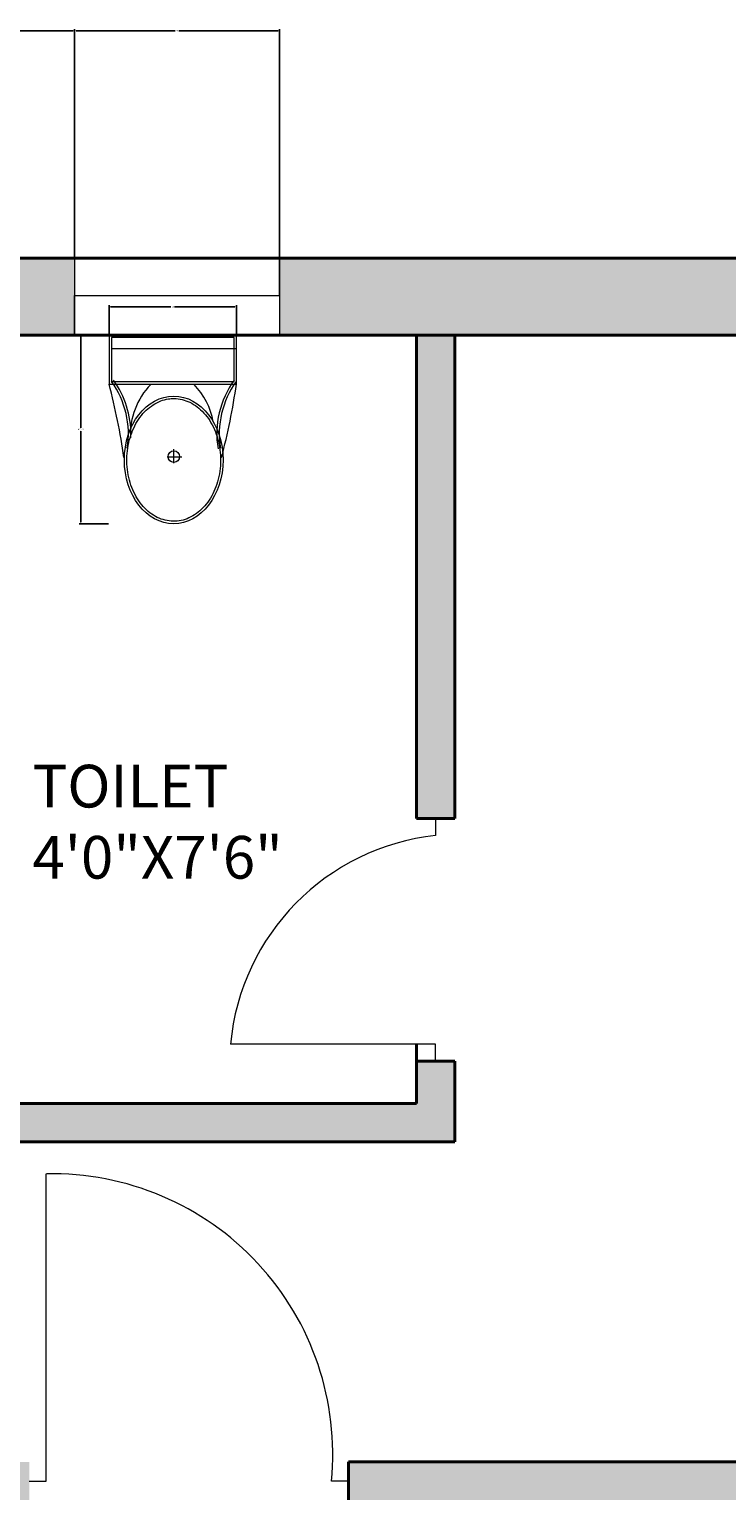
# Model space of a CAD drawing. Units: inches. Extents: x 1441 to 2460, y 1648 to 2683.
# Tile 21 of 35: x 1711 to 1792, y 2154 to 2326. Entities that reach past the tile are written whole.
import ezdxf

# ---------------------------------------------------------------- set-up
doc = ezdxf.new("R2010")
doc.units = ezdxf.units.IN
for name, color, linetype, lineweight in [('A-ANNO-DIMS', 2, 'Continuous', 18), ('A-AREA-IDEN', 7, 'Continuous', 20), ('A-DOOR', 3, 'Continuous', 20), ('A-FLOR-FIXT', 9, 'Continuous', 18), ('A-GLAZ', 4, 'Continuous', 18), ('A-WALL', 7, 'Continuous', 40)]:
    doc.layers.add(name, color=color, linetype=linetype, lineweight=lineweight)
doc.layers.add('A-WALL-PATT', color=251, linetype='Continuous', lineweight=13, true_color=0x636466)
doc.styles.get("Standard").update_dxf_attribs({"font": 'arial.ttf'})
doc.dimstyles.get("Standard").update_dxf_attribs({"dimtxt": 0.18, "dimasz": 0.18, "dimexe": 0.18, "dimexo": 0.0625, "dimgap": 0.09, "dimtad": 0, "dimtih": 1, "dimtoh": 1, "dimdec": 4, "dimzin": 0, "dimdsep": 46, "dimtxsty": 'Standard', "dimcen": 0.09, "dimadec": 0, "dimazin": 0, "dimtfac": 1, "dimtdec": 4, "dimtofl": 0, "dimtmove": 0, "dimatfit": 3, "dimfxl": 1, "dimtolj": 1, "dimtzin": 0, "dimarcsym": 0})

# ---------------------------------------------------------------- blocks, each defined once
blk = doc.blocks.new('A$C31115884')
for p, q in [((283.1, 497.7), (223.4, 497.7)), ((257.5, 466.4), (257.5, 523.2)), ((0, 200), (0, 0)), ((520, 200), (0, 200)), ((10, 190), (10, 10)), ((510, 190), (10, 190)), ((510, 10), (510, 190)), ((520, 0), (520, 200)), ((510, 54.5), (0, 54.5)), ((10, 10), (510, 10)), ((0, 0), (520, 0))]:
    blk.add_line(p, q)
blk.add_circle((255.6, 496.4), 23.6)
for centre, radius, start, end in [((2777.7, -204.6), 2807, 165.4549, 171.71327), ((3237, 905), 2807, 188.28673, 194.5451), ((-294.5, 403.3), 364.7, 324.20913, 9.34987), ((-294.5, 403.3), 374.7, 324.20913, 9.34987), ((139.5, 406.2), 293.5, 315.84364, 2.65635), ((805.8, 403.3), 364.7, 170.65013, 215.79087), ((805.8, 403.3), 374.7, 179.20365, 215.79087), ((383.6, 406.2), 293.5, 190.27735, 224.15636)]:
    blk.add_arc(centre, radius, start, end)
blk.add_ellipse((256.2, 509.9), major_axis=(0, -260.7), ratio=0.772727)
blk.add_open_spline([(256.2, 259.2), (263.1, 259.2), (270, 259.7), (287.8, 262.3), (298.7, 265.1), (319.9, 273.1), (330.2, 278.4), (350.1, 291.1), (359.7, 298.7), (377.7, 315.9), (386.2, 325.5), (401.7, 346.6), (408.8, 358.1), (421.3, 382.5), (426.8, 395.5), (435.9, 422.4), (439.5, 436.4), (444.8, 465.1), (446.5, 479.7), (447.9, 509.2), (447.6, 524), (445, 553.3), (442.7, 567.8), (436.3, 596), (432.1, 609.7), (421.9, 636), (416, 648.6), (402.5, 672.1), (395, 683), (378.6, 703), (369.8, 712.1), (351.1, 728), (341.3, 734.8), (320.9, 746.2), (310.4, 750.7), (288.9, 757.3), (278, 759.4), (256, 761), (245, 760.6), (223.1, 757.2), (212.3, 754.3), (191.1, 746.1), (180.8, 740.7), (160.9, 727.8), (151.4, 720.1), (133.5, 702.7), (125.1, 693), (109.6, 671.7), (102.6, 660.2), (90.2, 635.7), (84.9, 622.7), (76, 595.6), (72.4, 581.6), (67.2, 552.9), (65.6, 538.2), (64.4, 508.8), (64.8, 494), (67.5, 464.7), (69.9, 450.2), (76.6, 422), (80.8, 408.3), (91.1, 382.2), (97.2, 369.7), (110.8, 346.3), (118.4, 335.4), (134.8, 315.6), (143.7, 306.7), (162.4, 290.9), (172.3, 284.2), (192.8, 273), (203.3, 268.6), (224.8, 262.2), (235.8, 260.2), (249.9, 259.3), (253, 259.2), (256.2, 259.2)], degree=3, knots=[0, 0, 0, 0, 0.110105, 0.110105, 0.285049, 0.285049, 0.459994, 0.459994, 0.634938, 0.634938, 0.809882, 0.809882, 0.984827, 0.984827, 1.159771, 1.159771, 1.334715, 1.334715, 1.50966, 1.50966, 1.684604, 1.684604, 1.859549, 1.859549, 2.034493, 2.034493, 2.209437, 2.209437, 2.384382, 2.384382, 2.559326, 2.559326, 2.73427, 2.73427, 2.909215, 2.909215, 3.084159, 3.084159, 3.259103, 3.259103, 3.434048, 3.434048, 3.608992, 3.608992, 3.783936, 3.783936, 3.958881, 3.958881, 4.133825, 4.133825, 4.30877, 4.30877, 4.483714, 4.483714, 4.658658, 4.658658, 4.833603, 4.833603, 5.008547, 5.008547, 5.183491, 5.183491, 5.358436, 5.358436, 5.53338, 5.53338, 5.708324, 5.708324, 5.883269, 5.883269, 6.058213, 6.058213, 6.233158, 6.233158, 6.283185, 6.283185, 6.283185, 6.283185])
blk = doc.blocks.new('DOOR-BED1-36')
for p, q in [((2, 0), (2, 36)), ((0, 0), (2, 0)), ((37.39, 0), (35.39, 0))]:
    blk.add_line(p, q)
blk.add_arc((2.69, 3.15), 32.85, 354.488, 91.1985)
blk = doc.blocks.new('DOOR-WC-NORTH-24')
for p, q in [((24, 28.42), (24, 26.42)), ((24, 2), (0, 2)), ((24, 0), (24, 2))]:
    blk.add_line(p, q)
blk.add_arc((26.92, -0.45), 27.04, 96.2058, 174.7965)
blk = doc.blocks.new('*D34')
at = {"layer": 'A-ANNO-DIMS', "color": 0, "lineweight": -2, "transparency": 16777216}
for p, q in [((1719.85, 2289.7), (1716.42, 2289.7)), ((1716.6, 2289.52), (1716.6, 2278.83)), ((1716.6, 2267.78), (1716.6, 2278.46)), ((1719.85, 2267.6), (1716.42, 2267.6))]:
    blk.add_line(p, q, dxfattribs=at)
at = {"layer": 'A-ANNO-DIMS', "color": 0, "transparency": 16777216}
for points in [[(1716.57, 2289.52), (1716.63, 2289.52), (1716.6, 2289.7)], [(1716.57, 2267.78), (1716.63, 2267.78), (1716.6, 2267.6)]]:
    blk.add_solid(points, dxfattribs=at)
at = {"layer": 'Defpoints', "color": 0, "transparency": 16777216}
for p in [(1719.91, 2289.7), (1716.6, 2267.6), (1719.91, 2267.6)]:
    blk.add_point(p, dxfattribs=at)
at = {"layer": 'A-ANNO-DIMS', "color": 0, "transparency": 16777216, "insert": (1716.6, 2278.65), "char_height": 0.18, "attachment_point": 5}
blk.add_mtext('\\A1;WC 22', dxfattribs=at)
blk = doc.blocks.new('*D35')
at = {"layer": 'A-ANNO-DIMS', "color": 0, "lineweight": -2, "transparency": 16777216}
for p, q in [((1719.91, 2289.76), (1719.91, 2293.19)), ((1720.09, 2293.01), (1727.15, 2293.01)), ((1734.64, 2293.01), (1727.58, 2293.01)), ((1734.82, 2289.76), (1734.82, 2293.19))]:
    blk.add_line(p, q, dxfattribs=at)
at = {"layer": 'A-ANNO-DIMS', "color": 0, "transparency": 16777216}
for points in [[(1720.09, 2293.04), (1720.09, 2292.98), (1719.91, 2293.01)], [(1734.64, 2293.04), (1734.64, 2292.98), (1734.82, 2293.01)]]:
    blk.add_solid(points, dxfattribs=at)
at = {"layer": 'Defpoints', "color": 0, "transparency": 16777216}
for p in [(1719.91, 2293.01), (1719.91, 2289.7), (1734.82, 2289.7)]:
    blk.add_point(p, dxfattribs=at)
at = {"layer": 'A-ANNO-DIMS', "color": 0, "transparency": 16777216, "insert": (1727.37, 2293.01), "char_height": 0.18, "attachment_point": 5}
blk.add_mtext('\\A1;15', dxfattribs=at)
blk = doc.blocks.new('*D67')
at = {"layer": 'A-ANNO-DIMS', "color": 0, "lineweight": -2, "transparency": 16777216}
for p, q in [((1889.45, 2298.7), (1916.22, 2298.7)), ((1916.04, 2298.52), (1916.04, 2055.94)), ((1916.04, 1813), (1916.04, 2055.57)), ((1758.22, 1812.82), (1916.22, 1812.82))]:
    blk.add_line(p, q, dxfattribs=at)
at = {"layer": 'A-ANNO-DIMS', "color": 0, "transparency": 16777216}
for points in [[(1916.01, 2298.52), (1916.07, 2298.52), (1916.04, 2298.7)], [(1916.01, 1813), (1916.07, 1813), (1916.04, 1812.82)]]:
    blk.add_solid(points, dxfattribs=at)
at = {"layer": 'Defpoints', "color": 0, "transparency": 16777216}
for p in [(1889.39, 2298.7), (1916.04, 2298.7), (1758.16, 1812.82)]:
    blk.add_point(p, dxfattribs=at)
at = {"layer": 'A-ANNO-DIMS', "color": 0, "transparency": 16777216, "insert": (1916.04, 2055.76), "char_height": 0.18, "attachment_point": 5}
blk.add_mtext('\\A1;485.9', dxfattribs=at)
blk = doc.blocks.new('*D72')
at = {"layer": 'A-ANNO-DIMS', "color": 0, "lineweight": -2, "transparency": 16777216}
for p, q in [((1699.58, 2298.76), (1699.58, 2325.53)), ((1699.76, 2325.35), (1707.27, 2325.35)), ((1715.69, 2325.35), (1708.18, 2325.35)), ((1715.87, 2298.76), (1715.87, 2325.53))]:
    blk.add_line(p, q, dxfattribs=at)
at = {"layer": 'A-ANNO-DIMS', "color": 0, "transparency": 16777216}
for points in [[(1699.76, 2325.38), (1699.76, 2325.32), (1699.58, 2325.35)], [(1715.69, 2325.38), (1715.69, 2325.32), (1715.87, 2325.35)]]:
    blk.add_solid(points, dxfattribs=at)
at = {"layer": 'Defpoints', "color": 0, "transparency": 16777216}
for p in [(1715.87, 2325.35), (1699.58, 2298.7), (1715.87, 2298.7)]:
    blk.add_point(p, dxfattribs=at)
at = {"layer": 'A-ANNO-DIMS', "color": 0, "transparency": 16777216, "insert": (1707.72, 2325.35), "char_height": 0.18, "attachment_point": 5}
blk.add_mtext('\\A1;16.294', dxfattribs=at)
blk = doc.blocks.new('*D73')
at = {"layer": 'A-ANNO-DIMS', "color": 0, "lineweight": -2, "transparency": 16777216}
for p, q in [((1715.87, 2298.76), (1715.87, 2325.53)), ((1716.05, 2325.35), (1727.65, 2325.35)), ((1739.69, 2325.35), (1728.09, 2325.35)), ((1739.87, 2298.76), (1739.87, 2325.53))]:
    blk.add_line(p, q, dxfattribs=at)
at = {"layer": 'A-ANNO-DIMS', "color": 0, "transparency": 16777216}
for points in [[(1716.05, 2325.38), (1716.05, 2325.32), (1715.87, 2325.35)], [(1739.69, 2325.38), (1739.69, 2325.32), (1739.87, 2325.35)]]:
    blk.add_solid(points, dxfattribs=at)
at = {"layer": 'Defpoints', "color": 0, "transparency": 16777216}
for p in [(1739.87, 2325.35), (1715.87, 2298.7), (1739.87, 2298.7)]:
    blk.add_point(p, dxfattribs=at)
at = {"layer": 'A-ANNO-DIMS', "color": 0, "transparency": 16777216, "insert": (1727.87, 2325.35), "char_height": 0.18, "attachment_point": 5}
blk.add_mtext('\\A1;24', dxfattribs=at)

msp = doc.modelspace()

# ---------------------------------------------------------------- hatches: boundary and pattern name
at = {"layer": 'A-WALL-PATT'}
h = msp.add_hatch(color=256, dxfattribs=at)
h.dxf.hatch_style = 1
h.paths.add_polyline_path([(1627.5085, 2298.6952), (1568.8859, 2298.6952), (1568.8859, 2246.9605), (1577.8859, 2246.9605), (1577.8859, 2289.6952), (1627.5085, 2289.6952), (1627.5085, 2294.1952)])
h.paths.add_polyline_path([(1675.5777, 2298.6952), (1651.5085, 2298.6952), (1651.5085, 2289.6952), (1675.5777, 2289.6952), (1675.5777, 2294.1952)])
h.paths.add_polyline_path([(1667.3859, 2289.6952), (1662.8859, 2289.6952), (1662.8859, 2233.0622), (1667.3859, 2233.0622)])
h.paths.add_polyline_path([(1715.8721, 2294.3362), (1715.8721, 2295.2788), (1715.8721, 2298.6952), (1699.5777, 2298.6952), (1699.5777, 2289.6952), (1715.8721, 2289.6952)])
h.paths.add_polyline_path([(1707.8859, 2289.6952), (1703.3859, 2289.6952), (1703.3859, 2199.6952), (1707.8859, 2199.6952)])
h.paths.add_polyline_path([(1760.3859, 2204.637), (1755.8859, 2204.637), (1755.8859, 2199.6952), (1667.3859, 2199.6952), (1667.3859, 2204.637), (1662.8859, 2204.637), (1662.8859, 2195.1952), (1760.3859, 2195.1952)])
h.paths.add_polyline_path([(1760.3859, 2289.6952), (1755.8859, 2289.6952), (1755.8859, 2233.0622), (1760.3859, 2233.0622)])
h.paths.add_polyline_path([(1889.3859, 2298.6952), (1739.8721, 2298.6952), (1739.8721, 2289.6952), (1880.3859, 2289.6952), (1880.3859, 2250.8051), (1889.3859, 2250.8051)])
h.paths.add_polyline_path([(1889.3859, 2202.8051), (1880.3859, 2202.8051), (1880.3859, 2157.6952), (1747.948, 2157.6952), (1747.948, 2153.1952), (1755.8859, 2153.1952), (1755.8859, 2058.005), (1760.3859, 2058.005), (1760.3859, 2153.1952), (1880.3859, 2153.1952), (1880.3859, 2124.108), (1889.3859, 2124.108)])
h.paths.add_polyline_path([(1889.3859, 1984.8305), (1880.3859, 1984.8305), (1880.3859, 1834.1952), (1889.3859, 1834.1952)])
h.paths.add_polyline_path([(1889.3859, 2076.108), (1880.3859, 2076.108), (1880.3859, 2008.8305), (1889.3859, 2008.8305)])
h.paths.add_polyline_path([(1880.3859, 2027.1952), (1800.8859, 2027.1952), (1800.8859, 2000.9452), (1805.3859, 2000.9452), (1805.3859, 2022.6952), (1880.3859, 2022.6952)])
h.paths.add_polyline_path([(1800.8859, 2027.1952), (1760.3859, 2027.1952), (1760.3859, 2030.7912), (1755.8859, 2030.7912), (1755.8859, 2022.6952), (1800.8859, 2022.6952)])
h.paths.add_polyline_path([(1880.3859, 1974.6952), (1805.3859, 1974.6952), (1805.3859, 1978.7973), (1800.8859, 1978.7973), (1800.8859, 1974.6952), (1794.8823, 1974.6952), (1794.8823, 1970.1952), (1800.8859, 1970.1952), (1805.3859, 1970.1952), (1880.3859, 1970.1952)])
h.paths.add_polyline_path([(1760.3859, 1974.6952), (1755.8859, 1974.6952), (1755.8859, 1925.6952), (1751.8616, 1925.6952), (1751.8616, 1921.1952), (1760.3859, 1921.1952)])
h.paths.add_polyline_path([(1760.3859, 1921.1952), (1755.8859, 1921.1952), (1755.8859, 1843.1952), (1760.3859, 1843.1952)])
h.paths.add_polyline_path([(1799.1136, 1838.6952), (1799.1136, 1843.1952), (1760.3859, 1843.1952), (1751.8944, 1843.1952), (1751.8944, 1834.1952), (1758.1615, 1834.1952), (1799.1136, 1834.1952)])
h.paths.add_polyline_path([(1880.3859, 1843.1952), (1859.1136, 1843.1952), (1859.1136, 1834.1952), (1880.3859, 1834.1952)])
h.paths.add_polyline_path([(1577.8859, 1857.7914), (1568.8859, 1857.7914), (1568.8859, 1834.1952), (1695.0034, 1834.1952), (1695.0034, 1838.6952), (1695.0034, 1843.1952), (1577.8859, 1843.1952)])
h.paths.add_polyline_path([(1577.8859, 1959.2399), (1573.3859, 1959.2399), (1568.8859, 1959.2399), (1568.8859, 1905.7914), (1577.8859, 1905.7914), (1577.8859, 1921.1952), (1703.3859, 1921.1952), (1707.8859, 1921.1952), (1715.1501, 1921.1952), (1715.1501, 1925.6952), (1707.8859, 1925.6952), (1703.3859, 1925.6952), (1577.8859, 1925.6952)])
h.paths.add_polyline_path([(1577.8859, 2106.6907), (1568.8859, 2106.6907), (1568.8859, 2019.2399), (1577.8859, 2019.2399)])
h.paths.add_polyline_path([(1707.8859, 2051.6952), (1703.3859, 2051.6952), (1703.3859, 2048.6952), (1703.3859, 1925.6952), (1707.8859, 1925.6952)])
h.paths.add_polyline_path([(1703.3859, 2051.6952), (1676.3859, 2051.6952), (1676.3859, 2048.6952), (1703.3859, 2048.6952)])
h.paths.add_polyline_path([(1703.3859, 2102.6952), (1676.3859, 2102.6952), (1676.3859, 2099.6952), (1685.3859, 2099.6952), (1703.3859, 2099.6952)])
h.paths.add_polyline_path([(1707.8859, 2153.1952), (1710.5611, 2153.1952), (1710.5611, 2157.6952), (1707.8859, 2157.6952), (1707.8859, 2195.1952), (1703.3859, 2195.1952), (1703.3859, 2099.6952), (1707.8859, 2099.6952)])
h.paths.add_polyline_path([(1577.8859, 2198.9605), (1568.8859, 2198.9605), (1568.8859, 2166.6907), (1577.8859, 2166.6907)])

# ---------------------------------------------------------------- linework, layer by layer
at = {"layer": 'A-GLAZ'}
for p, q in [((1715.8721, 2298.6952), (1715.8721, 2295.2788)), ((1739.8721, 2294.3362), (1739.8721, 2298.6952)), ((1739.8721, 2298.6952), (1739.8721, 2289.6952)), ((1715.8721, 2295.2788), (1715.8721, 2289.6952)), ((1715.8721, 2289.6952), (1715.8721, 2294.3362)), ((1715.8721, 2294.3362), (1739.8721, 2294.3362))]:
    msp.add_line(p, q, dxfattribs=at)
at = {"layer": 'A-WALL'}
for p, q in [((1568.8859, 2298.6952), (1889.3859, 2298.6952)), ((1577.8859, 2289.6952), (1880.3859, 2289.6952)), ((1755.8859, 2289.6952), (1755.8859, 2233.0622)), ((1760.3859, 2289.6952), (1760.3859, 2233.0622)), ((1755.8859, 2233.0622), (1760.3859, 2233.0622)), ((1755.8859, 2206.637), (1755.8859, 2199.6952)), ((1760.3859, 2204.637), (1755.8859, 2204.637)), ((1760.3859, 2204.637), (1760.3859, 2195.1952)), ((1667.3859, 2199.6952), (1755.8859, 2199.6952)), ((1662.8859, 2195.1952), (1760.3859, 2195.1952)), ((1747.948, 2157.6952), (1747.948, 2153.1952)), ((1747.948, 2157.6952), (1880.3859, 2157.6952))]:
    msp.add_line(p, q, dxfattribs=at)

# ---------------------------------------------------------------- block references
at = {"layer": 'A-DOOR'}
for name, p in [('DOOR-WC-NORTH-24', (1734.14, 2204.64)), ('DOOR-BED1-36', (1710.56, 2155.45))]:
    msp.add_blockref(name, p, dxfattribs=at)
at = {"layer": 'A-FLOR-FIXT', "xscale": 0.0286729940675919, "yscale": 0.0286729940675919, "zscale": 0.0286729940675919, "rotation": 180}
msp.add_blockref('A$C31115884', (1734.8207, 2289.6952), dxfattribs=at)

# ---------------------------------------------------------------- texts
at = {"layer": 'A-AREA-IDEN', "insert": (1710.9317, 2239.3606), "char_height": 5, "attachment_point": 1}
msp.add_mtext_dynamic_manual_height_columns('TOILET\\P4\'0"X7\'6"', width=85.554017, gutter_width=12.5, heights=[0], dxfattribs=at)

# ---------------------------------------------------------------- dimensions: what is measured, and where the dimension line sits
at = {"layer": 'A-ANNO-DIMS'}
for base, p1, p2, override, picture, middle in [((1715.8721, 2325.3452), (1699.5777, 2298.6952), (1715.8721, 2298.6952), {"dimdec": 3, "dimlfac": 1, "dimrnd": 0, "dimzin": 0, "dimdsep": 46, "dimlunit": 2}, '*D72', (1707.7249, 2325.3452)), ((1739.8721, 2325.3452), (1715.8721, 2298.6952), (1739.8721, 2298.6952), {"dimdec": 0, "dimlfac": 1, "dimrnd": 0, "dimzin": 0, "dimdsep": 46, "dimlunit": 2}, '*D73', (1727.8721, 2325.3452))]:
    dim = msp.add_linear_dim(base=base, p1=p1, p2=p2, dimstyle='Standard', override=override, dxfattribs=at)
    dim.commit()
    dim.dimension.update_dxf_attribs({"geometry": picture, "text_midpoint": middle})
for base, p1, p2, angle, override, picture, middle in [((1916.0359, 2298.6952), (1758.1615, 1812.8171), (1889.3859, 2298.6952), 90, {"dimdec": 1, "dimlfac": 1, "dimrnd": 0, "dimzin": 0, "dimdsep": 46, "dimlunit": 2}, '*D67', (1916.0359, 2055.7561)), ((1719.9107, 2293.0094), (1734.8207, 2289.6952), (1719.9107, 2289.6952), 180, {"dimdec": 0, "dimlfac": 1, "dimrnd": 0, "dimzin": 0, "dimdsep": 46, "dimlunit": 2}, '*D35', (1727.3657, 2293.0094))]:
    dim = msp.add_linear_dim(base=base, p1=p1, p2=p2, angle=angle, dimstyle='Standard', override=override, dxfattribs=at)
    dim.commit()
    dim.dimension.update_dxf_attribs({"geometry": picture, "text_midpoint": middle})
dim = msp.add_linear_dim(base=(1716.5966, 2267.6006), p1=(1719.9107, 2289.6952), p2=(1719.9107, 2267.6006), angle=270, text='WC <>', dimstyle='Standard', override={"dimdec": 0, "dimlfac": 1, "dimrnd": 0, "dimzin": 0, "dimdsep": 46, "dimlunit": 2}, dxfattribs=at)
dim.commit()
dim.dimension.update_dxf_attribs({"geometry": '*D34', "text_midpoint": (1716.5966, 2278.6479)})

doc.saveas('drawing.dxf')
